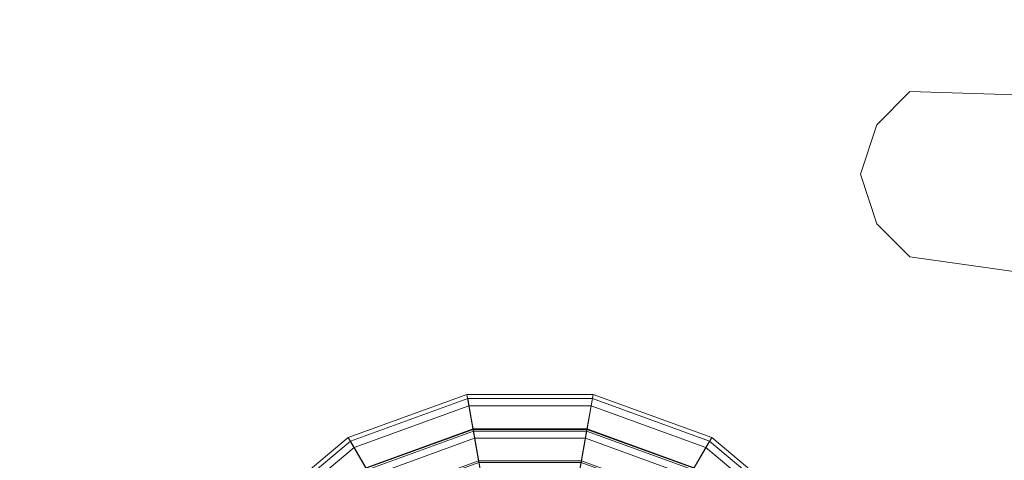
# Model space of a CAD drawing. Units: inches. Extents: x 375 to 1122, y 27 to 1069.
# Tile 143 of 155: x 731.16 to 734.829, y 900.205 to 901.848. Entities that reach past the tile are written whole.
import ezdxf

# ---------------------------------------------------------------- set-up
doc = ezdxf.new("R2010")
doc.units = ezdxf.units.IN
doc.layers.add('A-ANNO-DIMS', color=2, linetype='Continuous', lineweight=18)
doc.layers.add('Furniture', color=30, linetype='Continuous', lineweight=18)
doc.styles.get("Standard").update_dxf_attribs({"font": 'arial.ttf'})
doc.dimstyles.new('ISO-25', dxfattribs={"dimtxt": 12, "dimasz": 2.5, "dimexe": 1.5, "dimexo": 1.5, "dimtad": 1, "dimdec": 1, "dimlunit": 3, "dimtxsty": 'Standard', "dimblk": 'ARCHTICK', "dimcen": 2.5, "dimadec": 0, "dimazin": 0, "dimtfac": 1, "dimtdec": 1, "dimtmove": 0, "dimatfit": 3, "dimfxl": 1.5, "dimfxlon": 1, "dimarcsym": 0})

# ---------------------------------------------------------------- blocks, each defined once
blk = doc.blocks.new('A$C403C54AD')
for points, invisible_edges in [([(0.933982, 1.238319, -0.039653), (0.91859, 1.238319, -0.039653), (0.920129, 1.287573, -0.039653), (0.935521, 1.249093, -0.039653)], 5), ([(0.933982, 1.238319, -0.041193), (0.91859, 1.238319, -0.041193), (0.920129, 1.287573, -0.041193), (0.935521, 1.249093, -0.041193)], 5), ([(0.920129, 1.287573, -0.041193), (0.920129, 1.287573, -0.039653), (0.91859, 1.238319, -0.039653), (0.91859, 1.238319, -0.041193)], 5), ([(0.933982, 1.238319, -0.039653), (0.933982, 1.238319, -0.041193), (0.935521, 1.249093, -0.041193), (0.935521, 1.249093, -0.039653)], 5), ([(0.921668, 1.23524, -0.039653), (0.930903, 1.23524, -0.039653), (0.933982, 1.238319, -0.039653), (0.91859, 1.238319, -0.039653)], 5), ([(0.921668, 1.23524, -0.041193), (0.930903, 1.23524, -0.041193), (0.933982, 1.238319, -0.041193), (0.91859, 1.238319, -0.041193)], 5), ([(0.91859, 1.238319, -0.039653), (0.91859, 1.238319, -0.041193), (0.921668, 1.23524, -0.041193), (0.921668, 1.23524, -0.039653)], 5), ([(0.930903, 1.23524, -0.041193), (0.930903, 1.23524, -0.039653), (0.933982, 1.238319, -0.039653), (0.933982, 1.238319, -0.041193)], 5), ([(0.926286, 1.233701, -0.039653), (0.926286, 1.233701, -0.039653), (0.921668, 1.23524, -0.039653), (0.930903, 1.23524, -0.039653)], 4), ([(0.926286, 1.233701, -0.041193), (0.926286, 1.233701, -0.041193), (0.921668, 1.23524, -0.041193), (0.930903, 1.23524, -0.041193)], 4), ([(0.921668, 1.23524, -0.041193), (0.921668, 1.23524, -0.039653), (0.926286, 1.233701, -0.039653), (0.926286, 1.233701, -0.041193)], 1), ([(0.926286, 1.233701, -0.039653), (0.926286, 1.233701, -0.041193), (0.930903, 1.23524, -0.041193), (0.930903, 1.23524, -0.039653)], 4)]:
    blk.add_3dface(points, dxfattribs=dict(invisible_edges=invisible_edges))
for points in [[(0.958391, 1.228857, -0.04658), (0.980157, 1.202917, -0.043501), (0.980157, 1.202917, -0.043501), (0.950832, 1.219849, -0.04658)], [(0.96049, 1.226356, -0.043349), (0.958391, 1.228857, -0.04658), (0.950832, 1.219849, -0.04658), (0.95366, 1.218216, -0.043349)], [(0.960516, 1.226325, 0.116404), (0.958647, 1.228552, 0.10318), (0.951177, 1.219649, 0.10318), (0.953695, 1.218195, 0.116404)], [(0.958647, 1.228552, 0.10318), (0.959081, 1.228035, 0.074938), (0.951762, 1.219312, 0.074938), (0.951177, 1.219649, 0.10318)], [(0.959081, 1.228035, 0.074938), (0.96253, 1.223925, 0.056929), (0.956408, 1.216629, 0.056929), (0.951762, 1.219312, 0.074938)], [(0.950832, 1.219849, -0.04658), (0.980157, 1.202917, -0.043501), (0.980157, 1.202917, -0.043501), (0.94681, 1.208798, -0.04658)], [(0.95366, 1.218216, -0.043349), (0.950832, 1.219849, -0.04658), (0.94681, 1.208798, -0.04658), (0.950026, 1.20823, -0.043349)], [(0.953695, 1.218195, 0.116404), (0.951177, 1.219649, 0.10318), (0.947202, 1.208728, 0.10318), (0.950065, 1.208223, 0.116404)], [(0.951177, 1.219649, 0.10318), (0.951762, 1.219312, 0.074938), (0.947867, 1.208611, 0.074938), (0.947202, 1.208728, 0.10318)], [(0.951762, 1.219312, 0.074938), (0.956408, 1.216629, 0.056929), (0.95315, 1.20768, 0.056929), (0.947867, 1.208611, 0.074938)], [(0.967847, 1.210025, -0.040074), (0.95366, 1.218216, -0.043349), (0.950026, 1.20823, -0.043349), (0.966159, 1.205386, -0.040074)], [(0.958022, 1.215697, 0.12581), (0.953695, 1.218195, 0.116404), (0.950065, 1.208223, 0.116404), (0.954986, 1.207356, 0.12581)], [(0.953848, 1.218107, 0.102963), (0.956282, 1.216702, 0.115599), (0.953007, 1.207705, 0.115599), (0.95024, 1.208193, 0.102963)], [(0.954418, 1.217778, 0.075423), (0.953848, 1.218107, 0.102963), (0.95024, 1.208193, 0.102963), (0.950888, 1.208078, 0.075423)], [(0.958842, 1.215224, 0.058276), (0.954418, 1.217778, 0.075423), (0.950888, 1.208078, 0.075423), (0.955918, 1.207191, 0.058276)], [(0.94681, 1.208798, -0.04658), (0.980157, 1.202917, -0.043501), (0.980157, 1.202917, -0.043501), (0.94681, 1.197037, -0.04658)], [(0.950026, 1.20823, -0.043349), (0.94681, 1.208798, -0.04658), (0.94681, 1.197037, -0.04658), (0.950026, 1.197604, -0.043349)], [(0.950065, 1.208223, 0.116404), (0.947202, 1.208728, 0.10318), (0.947202, 1.197107, 0.10318), (0.950065, 1.197611, 0.116404)], [(0.947202, 1.208728, 0.10318), (0.947867, 1.208611, 0.074938), (0.947867, 1.197224, 0.074938), (0.947202, 1.197107, 0.10318)], [(0.947867, 1.208611, 0.074938), (0.95315, 1.20768, 0.056929), (0.95315, 1.198155, 0.056929), (0.947867, 1.197224, 0.074938)], [(0.966159, 1.205386, -0.040074), (0.950026, 1.20823, -0.043349), (0.950026, 1.197604, -0.043349), (0.966159, 1.200449, -0.040074)], [(0.954986, 1.207356, 0.12581), (0.950065, 1.208223, 0.116404), (0.950065, 1.197611, 0.116404), (0.954986, 1.198479, 0.12581)], [(0.95024, 1.208193, 0.102963), (0.953007, 1.207705, 0.115599), (0.953007, 1.19813, 0.115599), (0.95024, 1.197642, 0.102963)], [(0.950888, 1.208078, 0.075423), (0.95024, 1.208193, 0.102963), (0.95024, 1.197642, 0.102963), (0.950888, 1.197756, 0.075423)], [(0.955918, 1.207191, 0.058276), (0.950888, 1.208078, 0.075423), (0.950888, 1.197756, 0.075423), (0.955918, 1.198643, 0.058276)], [(0.94681, 1.197037, -0.04658), (0.980157, 1.202917, -0.043501), (0.980157, 1.202917, -0.043501), (0.950832, 1.185986, -0.04658)], [(0.950832, 1.185986, -0.04658), (0.980157, 1.202917, -0.043501), (0.980157, 1.202917, -0.043501), (0.958391, 1.176977, -0.04658)], [(0.966159, 1.200449, -0.040074), (0.950026, 1.197604, -0.043349), (0.95366, 1.187619, -0.043349), (0.967847, 1.19581, -0.040074)], [(0.954986, 1.198479, 0.12581), (0.950065, 1.197611, 0.116404), (0.953695, 1.187639, 0.116404), (0.958022, 1.190138, 0.12581)], [(0.955918, 1.198643, 0.058276), (0.950888, 1.197756, 0.075423), (0.954418, 1.188057, 0.075423), (0.958842, 1.190611, 0.058276)], [(0.950026, 1.197604, -0.043349), (0.94681, 1.197037, -0.04658), (0.950832, 1.185986, -0.04658), (0.95366, 1.187619, -0.043349)], [(0.950065, 1.197611, 0.116404), (0.947202, 1.197107, 0.10318), (0.951177, 1.186186, 0.10318), (0.953695, 1.187639, 0.116404)], [(0.947867, 1.197224, 0.074938), (0.95315, 1.198155, 0.056929), (0.956408, 1.189206, 0.056929), (0.951762, 1.186523, 0.074938)], [(0.95024, 1.197642, 0.102963), (0.953007, 1.19813, 0.115599), (0.956282, 1.189133, 0.115599), (0.953848, 1.187728, 0.102963)], [(0.950888, 1.197756, 0.075423), (0.95024, 1.197642, 0.102963), (0.953848, 1.187728, 0.102963), (0.954418, 1.188057, 0.075423)], [(0.947202, 1.197107, 0.10318), (0.947867, 1.197224, 0.074938), (0.951762, 1.186523, 0.074938), (0.951177, 1.186186, 0.10318)], [(0.951762, 1.186523, 0.074938), (0.956408, 1.189206, 0.056929), (0.96253, 1.18191, 0.056929), (0.959081, 1.1778, 0.074938)], [(0.95366, 1.187619, -0.043349), (0.950832, 1.185986, -0.04658), (0.958391, 1.176977, -0.04658), (0.96049, 1.179479, -0.043349)], [(0.953695, 1.187639, 0.116404), (0.951177, 1.186186, 0.10318), (0.958647, 1.177283, 0.10318), (0.960516, 1.17951, 0.116404)], [(0.951177, 1.186186, 0.10318), (0.951762, 1.186523, 0.074938), (0.959081, 1.1778, 0.074938), (0.958647, 1.177283, 0.10318)]]:
    blk.add_3dface(points)
blk = doc.blocks.new('_ArchTick')
at = {"color": 0, "linetype": 'ByBlock', "const_width": 0.15}
blk.add_lwpolyline([(-0.5, -0.5), (0.5, 0.5)], dxfattribs=at)
blk = doc.blocks.new('*D73')
at = {"layer": 'A-ANNO-DIMS', "color": 0, "lineweight": -2, "transparency": 16777216}
for p, q in [((686.7573, 932.4277), (686.7573, 929.4277)), ((770.7573, 932.4277), (770.7573, 929.4277)), ((686.7573, 930.9277), (770.7573, 930.9277)), ((770.7573, 930.9277), (987.6096, 930.9277))]:
    blk.add_line(p, q, dxfattribs=at)
at = {"layer": 'Defpoints', "color": 0, "transparency": 16777216}
for p in [(686.7573, 943.5277), (770.7573, 943.5277), (770.7573, 930.9277)]:
    blk.add_point(p, dxfattribs=at)
at = {"layer": 'A-ANNO-DIMS', "color": 0, "lineweight": -2, "transparency": 16777216, "xscale": 2.5, "yscale": 2.5, "zscale": 2.5, "rotation": 180}
blk.add_blockref('_ArchTick', (686.7573, 930.9277), dxfattribs=at)
at = {"layer": 'A-ANNO-DIMS', "color": 0, "lineweight": -2, "transparency": 16777216, "xscale": 2.5, "yscale": 2.5, "zscale": 2.5}
blk.add_blockref('_ArchTick', (770.7573, 930.9277), dxfattribs=at)
at = {"layer": 'A-ANNO-DIMS', "color": 0, "transparency": 16777216, "insert": (880.4335, 937.7573), "char_height": 12, "attachment_point": 5}
blk.add_mtext('2-PANEL SLIDER 7\'-0" TYP.', dxfattribs=at)
blk = doc.blocks.new('*D88')
at = {"layer": 'A-ANNO-DIMS', "color": 0, "lineweight": -2, "transparency": 16777216}
for p, q in [((731.0073, 1052.5277), (731.0073, 1055.5277)), ((854.0073, 1052.5277), (854.0073, 1055.5277)), ((731.0073, 1054.0277), (854.0073, 1054.0277))]:
    blk.add_line(p, q, dxfattribs=at)
at = {"layer": 'Defpoints', "color": 0, "transparency": 16777216}
for p in [(854.0073, 1054.0277), (731.0073, 502.5277), (854.0073, 502.5277)]:
    blk.add_point(p, dxfattribs=at)
at = {"layer": 'A-ANNO-DIMS', "color": 0, "lineweight": -2, "transparency": 16777216, "xscale": 2.5, "yscale": 2.5, "zscale": 2.5, "rotation": 180}
blk.add_blockref('_ArchTick', (731.0073, 1054.0277), dxfattribs=at)
at = {"layer": 'A-ANNO-DIMS', "color": 0, "lineweight": -2, "transparency": 16777216, "xscale": 2.5, "yscale": 2.5, "zscale": 2.5}
blk.add_blockref('_ArchTick', (854.0073, 1054.0277), dxfattribs=at)
at = {"layer": 'A-ANNO-DIMS', "color": 0, "transparency": 16777216, "insert": (792.5073, 1060.7837), "char_height": 12, "attachment_point": 5}
blk.add_mtext('10\'-3"', dxfattribs=at)
blk = doc.blocks.new('*D91')
at = {"layer": 'A-ANNO-DIMS', "color": 0, "lineweight": -2, "transparency": 16777216}
for p, q in [((728.0073, 1052.5277), (728.0073, 1055.5277)), ((788.0073, 1052.5277), (788.0073, 1055.5277)), ((728.0073, 1054.0277), (788.0073, 1054.0277))]:
    blk.add_line(p, q, dxfattribs=at)
at = {"layer": 'Defpoints', "color": 0, "transparency": 16777216}
for p in [(788.0073, 1054.0277), (728.0073, 774.0277), (788.0073, 774.0277)]:
    blk.add_point(p, dxfattribs=at)
at = {"layer": 'A-ANNO-DIMS', "color": 0, "lineweight": -2, "transparency": 16777216, "xscale": 2.5, "yscale": 2.5, "zscale": 2.5, "rotation": 180}
blk.add_blockref('_ArchTick', (728.0073, 1054.0277), dxfattribs=at)
at = {"layer": 'A-ANNO-DIMS', "color": 0, "lineweight": -2, "transparency": 16777216, "xscale": 2.5, "yscale": 2.5, "zscale": 2.5}
blk.add_blockref('_ArchTick', (788.0073, 1054.0277), dxfattribs=at)
at = {"layer": 'A-ANNO-DIMS', "color": 0, "transparency": 16777216, "insert": (758.0073, 1060.7796), "char_height": 12, "attachment_point": 5}
blk.add_mtext('5\'-0"', dxfattribs=at)

msp = doc.modelspace()

# ---------------------------------------------------------------- block references
at = {"layer": 'Furniture', "xscale": 39.9918517141215, "yscale": 39.9918517141215, "zscale": 39.9918517141215, "rotation": 270}
msp.add_blockref('A$C403C54AD', (684.9549, 938.3156, 0.024), dxfattribs=at)

# ---------------------------------------------------------------- dimensions: what is measured, and where the dimension line sits
at = {"layer": 'A-ANNO-DIMS'}
for base, p1, p2, picture, middle in [((788.0073, 1054.0277), (728.0073, 774.0277), (788.0073, 774.0277), '*D91', (758.0073, 1060.7796)), ((854.0073, 1054.0277), (731.0073, 502.5277), (854.0073, 502.5277), '*D88', (792.5073, 1060.7837))]:
    dim = msp.add_linear_dim(base=base, p1=p1, p2=p2, dimstyle='ISO-25', override={"dimdec": 1, "dimlfac": 1, "dimrnd": 0, "dimzin": 1, "dimdsep": 46, "dimlunit": 4, "dimfrac": 2}, dxfattribs=at)
    dim.commit()
    dim.dimension.update_dxf_attribs({"geometry": picture, "text_midpoint": middle})
dim = msp.add_linear_dim(base=(770.7573, 930.9277), p1=(686.7573, 943.5277), p2=(770.7573, 943.5277), text='2-PANEL SLIDER <> TYP.', dimstyle='ISO-25', override={"dimdec": 1, "dimlfac": 1, "dimrnd": 0, "dimzin": 1, "dimdsep": 46, "dimlunit": 4, "dimfrac": 2}, dxfattribs=at)
dim.commit()
dim.dimension.update_dxf_attribs({"geometry": '*D73', "text_midpoint": (880.4335, 937.7573)})

doc.saveas('drawing.dxf')
